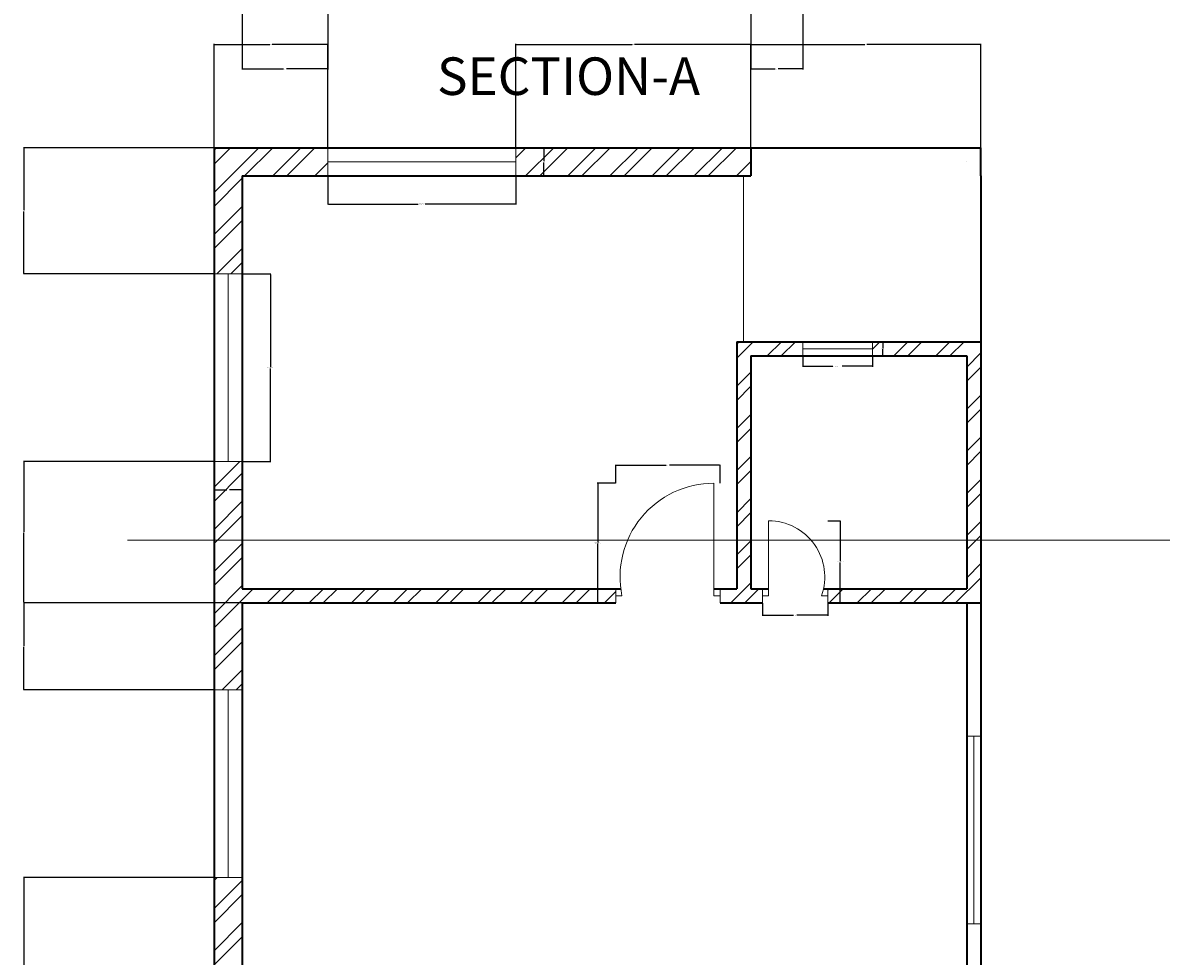
# Model space of a CAD drawing. Units: inches. Extents: x 1850 to 3445, y 1558 to 2756.
# Tile 10 of 13: x 2640 to 3003, y 1958 to 2256. Entities that reach past the tile are written whole.
import ezdxf

# ---------------------------------------------------------------- set-up
doc = ezdxf.new("R2010")
doc.units = ezdxf.units.IN
for name, color, linetype, lineweight in [('A-ANNO-DIMS', 2, 'Continuous', 18), ('A-ANNO-SYMB', 2, 'Continuous', 18), ('A-ANNO-TEXT', 7, 'Continuous', 18), ('A-DOOR', 3, 'Continuous', 18), ('A-GLAZ', 4, 'Continuous', 18), ('A-WALL', 7, 'Continuous', 35), ('A-WALL-PATT', 252, 'Continuous', 13)]:
    doc.layers.add(name, color=color, linetype=linetype, lineweight=lineweight)
doc.styles.get("Standard").update_dxf_attribs({"font": 'arial.ttf'})
doc.dimstyles.get("Standard").update_dxf_attribs({"dimtxt": 0.18, "dimasz": 0.18, "dimexe": 0.18, "dimexo": 0.0625, "dimgap": 0.09, "dimtad": 0, "dimtih": 1, "dimtoh": 1, "dimdec": 4, "dimzin": 0, "dimdsep": 46, "dimtxsty": 'Standard', "dimcen": 0.09, "dimadec": 0, "dimazin": 0, "dimtfac": 1, "dimtdec": 4, "dimtofl": 0, "dimtmove": 0, "dimatfit": 3, "dimfxl": 1, "dimtolj": 1, "dimtzin": 0, "dimarcsym": 0})

# ---------------------------------------------------------------- blocks, each defined once
blk = doc.blocks.new('WIN-60-W9')
for p, q in [((0, 9), (0, 0)), ((60, 4.5), (60, 9)), ((60, 9), (60, 0)), ((0, 0), (0, 4.5)), ((0, 4.5), (60, 4.5))]:
    blk.add_line(p, q)
blk = doc.blocks.new('WIN-60-W9-ALT')
for p, q in [((9, 60), (0, 60)), ((0, 60), (4.5, 60)), ((4.5, 60), (4.5, 0)), ((4.5, 0), (0, 0)), ((0, 0), (9, 0))]:
    blk.add_line(p, q)
blk = doc.blocks.new('WIN-60-W4_5')
for p, q in [((0, 60), (4.5, 60)), ((4.5, 60), (2.25, 60)), ((2.25, 60), (2.25, 0)), ((2.25, 0), (0, 0)), ((0, 0), (4.5, 0))]:
    blk.add_line(p, q)
blk = doc.blocks.new('WIN-BATH-GROUND')
for p, q in [((0, 0), (0, 4.5)), ((22.27, 2.25), (22.27, 4.5)), ((22.27, 4.5), (22.27, 0)), ((0, 2.25), (22.27, 2.25))]:
    blk.add_line(p, q)
blk = doc.blocks.new('DOOR-BATH-GROUND')
for p, q in [((2, 2.25), (2, 26.25)), ((0, 4.5), (0, 0)), ((20.9, 4.5), (20.9, 0)), ((0, 0), (0, 2.25)), ((0, 2.25), (2, 2.25)), ((20.9, 2.25), (18.9, 2.25)), ((20.9, 0), (20.9, 2.25))]:
    blk.add_line(p, q)
blk.add_arc((2, 8.3), 17.95, 340.2941, 90)
blk = doc.blocks.new('DOOR-BED-GROUND')
for p, q in [((31.38, 2.25), (31.38, 38.25)), ((0, 4.5), (0, 0)), ((33.38, 4.5), (33.38, 0)), ((0, 0), (0, 2.25)), ((0, 2.25), (2, 2.25)), ((33.38, 2.25), (31.38, 2.25)), ((33.38, 0), (33.38, 2.25))]:
    blk.add_line(p, q)
blk.add_arc((31.38, 8.26), 29.99, 90, 191.5706)
blk = doc.blocks.new('*D28')
at = {"layer": 'A-ANNO-DIMS', "color": 0, "lineweight": -2, "transparency": 16777216}
for p, q in [((2737.2, 2207.12), (2737.2, 2198)), ((2797.2, 2207.12), (2797.2, 2198)), ((2737.38, 2198.18), (2766.08, 2198.18)), ((2797.02, 2198.18), (2768.32, 2198.18))]:
    blk.add_line(p, q, dxfattribs=at)
at = {"layer": 'A-ANNO-DIMS', "color": 0, "transparency": 16777216}
for points in [[(2737.38, 2198.21), (2737.38, 2198.15), (2737.2, 2198.18)], [(2797.02, 2198.21), (2797.02, 2198.15), (2797.2, 2198.18)]]:
    blk.add_solid(points, dxfattribs=at)
at = {"layer": 'Defpoints', "color": 0, "transparency": 16777216}
for p in [(2737.2, 2207.18), (2797.2, 2207.18), (2797.2, 2198.18)]:
    blk.add_point(p, dxfattribs=at)
at = {"layer": 'A-ANNO-DIMS', "color": 0, "transparency": 16777216, "insert": (2767.2, 2198.18), "char_height": 0.18, "attachment_point": 5}
blk.add_mtext('\\A1;WINDOW 60 TYP.', dxfattribs=at)
blk = doc.blocks.new('*D29')
at = {"layer": 'A-ANNO-DIMS', "color": 0, "lineweight": -2, "transparency": 16777216}
for p, q in [((2797.26, 2216.18), (2806.38, 2216.18)), ((2806.2, 2216), (2806.2, 2211.87)), ((2806.2, 2207.36), (2806.2, 2211.5)), ((2797.26, 2207.18), (2806.38, 2207.18))]:
    blk.add_line(p, q, dxfattribs=at)
at = {"layer": 'A-ANNO-DIMS', "color": 0, "transparency": 16777216}
for points in [[(2806.17, 2216), (2806.23, 2216), (2806.2, 2216.18)], [(2806.17, 2207.36), (2806.23, 2207.36), (2806.2, 2207.18)]]:
    blk.add_solid(points, dxfattribs=at)
at = {"layer": 'Defpoints', "color": 0, "transparency": 16777216}
for p in [(2797.2, 2216.18), (2806.2, 2216.18), (2797.2, 2207.18)]:
    blk.add_point(p, dxfattribs=at)
at = {"layer": 'A-ANNO-DIMS', "color": 0, "transparency": 16777216, "insert": (2806.2, 2211.68), "char_height": 0.18, "attachment_point": 5}
blk.add_mtext('\\A1;9 TYP.', dxfattribs=at)
blk = doc.blocks.new('*D32')
at = {"layer": 'A-ANNO-DIMS', "color": 0, "lineweight": -2, "transparency": 16777216}
for p, q in [((2709.88, 2175.83), (2719, 2175.83)), ((2718.82, 2175.65), (2718.82, 2146.01)), ((2718.82, 2116.01), (2718.82, 2145.65)), ((2709.88, 2115.83), (2719, 2115.83))]:
    blk.add_line(p, q, dxfattribs=at)
at = {"layer": 'A-ANNO-DIMS', "color": 0, "transparency": 16777216}
for points in [[(2718.79, 2175.65), (2718.85, 2175.65), (2718.82, 2175.83)], [(2718.79, 2116.01), (2718.85, 2116.01), (2718.82, 2115.83)]]:
    blk.add_solid(points, dxfattribs=at)
at = {"layer": 'Defpoints', "color": 0, "transparency": 16777216}
for p in [(2709.82, 2175.83), (2718.82, 2175.83), (2709.82, 2115.83)]:
    blk.add_point(p, dxfattribs=at)
at = {"layer": 'A-ANNO-DIMS', "color": 0, "transparency": 16777216, "insert": (2718.82, 2145.83), "char_height": 0.18, "attachment_point": 5}
blk.add_mtext('\\A1;WINDOW 60 TYP.', dxfattribs=at)
blk = doc.blocks.new('*D33')
at = {"layer": 'A-ANNO-DIMS', "color": 0, "lineweight": -2, "transparency": 16777216}
for p, q in [((2700.82, 2115.77), (2700.82, 2106.65)), ((2709.82, 2115.77), (2709.82, 2106.65)), ((2701, 2106.83), (2704.86, 2106.83)), ((2709.64, 2106.83), (2705.78, 2106.83))]:
    blk.add_line(p, q, dxfattribs=at)
at = {"layer": 'A-ANNO-DIMS', "color": 0, "transparency": 16777216}
for points in [[(2701, 2106.86), (2701, 2106.8), (2700.82, 2106.83)], [(2709.64, 2106.86), (2709.64, 2106.8), (2709.82, 2106.83)]]:
    blk.add_solid(points, dxfattribs=at)
at = {"layer": 'Defpoints', "color": 0, "transparency": 16777216}
for p in [(2700.82, 2115.83), (2709.82, 2115.83), (2709.82, 2106.83)]:
    blk.add_point(p, dxfattribs=at)
at = {"layer": 'A-ANNO-DIMS', "color": 0, "transparency": 16777216, "insert": (2705.32, 2106.83), "char_height": 0.18, "attachment_point": 5}
blk.add_mtext('\\A1;9 TYP.', dxfattribs=at)
blk = doc.blocks.new('*D44')
at = {"layer": 'A-ANNO-DIMS', "color": 0, "lineweight": -2, "transparency": 16777216}
for p, q in [((2888.9, 2149.62), (2888.9, 2146.16)), ((2889.08, 2146.34), (2898.55, 2146.34)), ((2910.99, 2146.34), (2901.51, 2146.34)), ((2911.17, 2149.62), (2911.17, 2146.16))]:
    blk.add_line(p, q, dxfattribs=at)
at = {"layer": 'A-ANNO-DIMS', "color": 0, "transparency": 16777216}
for points in [[(2889.08, 2146.37), (2889.08, 2146.31), (2888.9, 2146.34)], [(2910.99, 2146.37), (2910.99, 2146.31), (2911.17, 2146.34)]]:
    blk.add_solid(points, dxfattribs=at)
at = {"layer": 'Defpoints', "color": 0, "transparency": 16777216}
for p in [(2888.9, 2149.68), (2911.17, 2149.68), (2911.17, 2146.34)]:
    blk.add_point(p, dxfattribs=at)
at = {"layer": 'A-ANNO-DIMS', "color": 0, "transparency": 16777216, "insert": (2900.03, 2146.34), "char_height": 0.18, "attachment_point": 5}
blk.add_mtext('\\A1;BATH WINDOW 22 TYP.', dxfattribs=at)
blk = doc.blocks.new('*D45')
at = {"layer": 'A-ANNO-DIMS', "color": 0, "lineweight": -2, "transparency": 16777216}
for p, q in [((2911.23, 2154.18), (2914.69, 2154.18)), ((2914.51, 2154), (2914.51, 2152.12)), ((2914.51, 2149.86), (2914.51, 2151.75)), ((2911.23, 2149.68), (2914.69, 2149.68))]:
    blk.add_line(p, q, dxfattribs=at)
at = {"layer": 'A-ANNO-DIMS', "color": 0, "transparency": 16777216}
for points in [[(2914.48, 2154), (2914.54, 2154), (2914.51, 2154.18)], [(2914.48, 2149.86), (2914.54, 2149.86), (2914.51, 2149.68)]]:
    blk.add_solid(points, dxfattribs=at)
at = {"layer": 'Defpoints', "color": 0, "transparency": 16777216}
for p in [(2911.17, 2154.18), (2914.51, 2154.18), (2911.17, 2149.68)]:
    blk.add_point(p, dxfattribs=at)
at = {"layer": 'A-ANNO-DIMS', "color": 0, "transparency": 16777216, "insert": (2914.51, 2151.93), "char_height": 0.18, "attachment_point": 5}
blk.add_mtext('\\A1;5 TYP.', dxfattribs=at)
blk = doc.blocks.new('*D56')
at = {"layer": 'A-ANNO-DIMS', "color": 0, "lineweight": -2, "transparency": 16777216}
for p, q in [((2896.98, 2096.93), (2901.03, 2096.93)), ((2900.85, 2096.75), (2900.85, 2083.99)), ((2900.85, 2070.86), (2900.85, 2083.63)), ((2896.98, 2070.68), (2901.03, 2070.68))]:
    blk.add_line(p, q, dxfattribs=at)
at = {"layer": 'A-ANNO-DIMS', "color": 0, "transparency": 16777216}
for points in [[(2900.82, 2096.75), (2900.88, 2096.75), (2900.85, 2096.93)], [(2900.82, 2070.86), (2900.88, 2070.86), (2900.85, 2070.68)]]:
    blk.add_solid(points, dxfattribs=at)
at = {"layer": 'Defpoints', "color": 0, "transparency": 16777216}
for p in [(2896.91, 2096.93), (2900.85, 2096.93), (2896.91, 2070.68)]:
    blk.add_point(p, dxfattribs=at)
at = {"layer": 'A-ANNO-DIMS', "color": 0, "transparency": 16777216, "insert": (2900.85, 2083.81), "char_height": 0.18, "attachment_point": 5}
blk.add_mtext('\\A1;BATH DOOR 26 TYP.', dxfattribs=at)
blk = doc.blocks.new('*D57')
at = {"layer": 'A-ANNO-DIMS', "color": 0, "lineweight": -2, "transparency": 16777216}
for p, q in [((2876.02, 2070.62), (2876.02, 2066.57)), ((2896.91, 2070.62), (2896.91, 2066.57)), ((2876.2, 2066.75), (2885.94, 2066.75)), ((2896.73, 2066.75), (2886.99, 2066.75))]:
    blk.add_line(p, q, dxfattribs=at)
at = {"layer": 'A-ANNO-DIMS', "color": 0, "transparency": 16777216}
for points in [[(2876.2, 2066.78), (2876.2, 2066.72), (2876.02, 2066.75)], [(2896.73, 2066.78), (2896.73, 2066.72), (2896.91, 2066.75)]]:
    blk.add_solid(points, dxfattribs=at)
at = {"layer": 'Defpoints', "color": 0, "transparency": 16777216}
for p in [(2876.02, 2070.68), (2896.91, 2070.68), (2896.91, 2066.75)]:
    blk.add_point(p, dxfattribs=at)
at = {"layer": 'A-ANNO-DIMS', "color": 0, "transparency": 16777216, "insert": (2886.47, 2066.75), "char_height": 0.18, "attachment_point": 5}
blk.add_mtext('\\A1;21 TYP.', dxfattribs=at)
blk = doc.blocks.new('*D58')
at = {"layer": 'A-ANNO-DIMS', "color": 0, "lineweight": -2, "transparency": 16777216}
for p, q in [((2829.09, 2108.93), (2823.24, 2108.93)), ((2823.42, 2108.75), (2823.42, 2089.99)), ((2823.42, 2070.86), (2823.42, 2089.63)), ((2829.09, 2070.68), (2823.24, 2070.68))]:
    blk.add_line(p, q, dxfattribs=at)
at = {"layer": 'A-ANNO-DIMS', "color": 0, "transparency": 16777216}
for points in [[(2823.39, 2108.75), (2823.45, 2108.75), (2823.42, 2108.93)], [(2823.39, 2070.86), (2823.45, 2070.86), (2823.42, 2070.68)]]:
    blk.add_solid(points, dxfattribs=at)
at = {"layer": 'Defpoints', "color": 0, "transparency": 16777216}
for p in [(2823.42, 2108.93), (2829.16, 2108.93), (2829.16, 2070.68)]:
    blk.add_point(p, dxfattribs=at)
at = {"layer": 'A-ANNO-DIMS', "color": 0, "transparency": 16777216, "insert": (2823.42, 2089.81), "char_height": 0.18, "attachment_point": 5}
blk.add_mtext('\\A1;BED DOOR 38 TYP.', dxfattribs=at)
blk = doc.blocks.new('*D59')
at = {"layer": 'A-ANNO-DIMS', "color": 0, "lineweight": -2, "transparency": 16777216}
for p, q in [((2829.16, 2109), (2829.16, 2114.85)), ((2829.34, 2114.67), (2845.32, 2114.67)), ((2862.35, 2114.67), (2846.37, 2114.67)), ((2862.53, 2109), (2862.53, 2114.85))]:
    blk.add_line(p, q, dxfattribs=at)
at = {"layer": 'A-ANNO-DIMS', "color": 0, "transparency": 16777216}
for points in [[(2829.34, 2114.7), (2829.34, 2114.64), (2829.16, 2114.67)], [(2862.35, 2114.7), (2862.35, 2114.64), (2862.53, 2114.67)]]:
    blk.add_solid(points, dxfattribs=at)
at = {"layer": 'Defpoints', "color": 0, "transparency": 16777216}
for p in [(2862.53, 2114.67), (2829.16, 2108.93), (2862.53, 2108.93)]:
    blk.add_point(p, dxfattribs=at)
at = {"layer": 'A-ANNO-DIMS', "color": 0, "transparency": 16777216, "insert": (2845.84, 2114.67), "char_height": 0.18, "attachment_point": 5}
blk.add_mtext('\\A1;33 TYP.', dxfattribs=at)
blk = doc.blocks.new('*D86')
at = {"layer": 'A-ANNO-DIMS', "color": 0, "lineweight": -2, "transparency": 16777216}
for p, q in [((2700.82, 2216.25), (2700.82, 2249.41)), ((2701, 2249.23), (2718.62, 2249.23)), ((2737.02, 2249.23), (2719.4, 2249.23)), ((2737.2, 2216.25), (2737.2, 2249.41))]:
    blk.add_line(p, q, dxfattribs=at)
at = {"layer": 'A-ANNO-DIMS', "color": 0, "transparency": 16777216}
for points in [[(2701, 2249.26), (2701, 2249.2), (2700.82, 2249.23)], [(2737.02, 2249.26), (2737.02, 2249.2), (2737.2, 2249.23)]]:
    blk.add_solid(points, dxfattribs=at)
at = {"layer": 'Defpoints', "color": 0, "transparency": 16777216}
for p in [(2737.2, 2249.23), (2700.82, 2216.18), (2737.2, 2216.18)]:
    blk.add_point(p, dxfattribs=at)
at = {"layer": 'A-ANNO-DIMS', "color": 0, "transparency": 16777216, "insert": (2719.01, 2249.23), "char_height": 0.18, "attachment_point": 5}
blk.add_mtext('\\A1;36.38', dxfattribs=at)
blk = doc.blocks.new('*D87')
at = {"layer": 'A-ANNO-DIMS', "color": 0, "lineweight": -2, "transparency": 16777216}
for p, q in [((2797.2, 2216.25), (2797.2, 2249.41)), ((2797.38, 2249.23), (2834.37, 2249.23)), ((2872.14, 2249.23), (2835.15, 2249.23)), ((2872.32, 2216.25), (2872.32, 2249.41))]:
    blk.add_line(p, q, dxfattribs=at)
at = {"layer": 'A-ANNO-DIMS', "color": 0, "transparency": 16777216}
for points in [[(2797.38, 2249.26), (2797.38, 2249.2), (2797.2, 2249.23)], [(2872.14, 2249.26), (2872.14, 2249.2), (2872.32, 2249.23)]]:
    blk.add_solid(points, dxfattribs=at)
at = {"layer": 'Defpoints', "color": 0, "transparency": 16777216}
for p in [(2872.32, 2249.23), (2797.2, 2216.18), (2872.32, 2216.18)]:
    blk.add_point(p, dxfattribs=at)
at = {"layer": 'A-ANNO-DIMS', "color": 0, "transparency": 16777216, "insert": (2834.76, 2249.23), "char_height": 0.18, "attachment_point": 5}
blk.add_mtext('\\A1;75.12', dxfattribs=at)
blk = doc.blocks.new('*D88')
at = {"layer": 'A-ANNO-DIMS', "color": 0, "lineweight": -2, "transparency": 16777216}
for p, q in [((2872.32, 2216.25), (2872.32, 2249.41)), ((2872.5, 2249.23), (2908.75, 2249.23)), ((2945.64, 2249.23), (2909.4, 2249.23)), ((2945.82, 2216.25), (2945.82, 2249.41))]:
    blk.add_line(p, q, dxfattribs=at)
at = {"layer": 'A-ANNO-DIMS', "color": 0, "transparency": 16777216}
for points in [[(2872.5, 2249.26), (2872.5, 2249.2), (2872.32, 2249.23)], [(2945.64, 2249.26), (2945.64, 2249.2), (2945.82, 2249.23)]]:
    blk.add_solid(points, dxfattribs=at)
at = {"layer": 'Defpoints', "color": 0, "transparency": 16777216}
for p in [(2945.82, 2249.23), (2872.32, 2216.18), (2945.82, 2216.18)]:
    blk.add_point(p, dxfattribs=at)
at = {"layer": 'A-ANNO-DIMS', "color": 0, "transparency": 16777216, "insert": (2909.07, 2249.23), "char_height": 0.18, "attachment_point": 5}
blk.add_mtext('\\A1;73.5', dxfattribs=at)
blk = doc.blocks.new('*D98')
at = {"layer": 'A-ANNO-DIMS', "color": 0, "lineweight": -2, "transparency": 16777216}
for p, q in [((2700.76, 1982.85), (2639.89, 1982.85)), ((2640.07, 1982.67), (2640.07, 1946.71)), ((2640.07, 1910.4), (2640.07, 1946.35)), ((2700.76, 1910.22), (2639.89, 1910.22))]:
    blk.add_line(p, q, dxfattribs=at)
at = {"layer": 'A-ANNO-DIMS', "color": 0, "transparency": 16777216}
for points in [[(2640.04, 1982.67), (2640.1, 1982.67), (2640.07, 1982.85)], [(2640.04, 1910.4), (2640.1, 1910.4), (2640.07, 1910.22)]]:
    blk.add_solid(points, dxfattribs=at)
at = {"layer": 'Defpoints', "color": 0, "transparency": 16777216}
for p in [(2640.07, 1982.85), (2700.82, 1982.85), (2700.82, 1910.22)]:
    blk.add_point(p, dxfattribs=at)
at = {"layer": 'A-ANNO-DIMS', "color": 0, "transparency": 16777216, "insert": (2640.07, 1946.53), "char_height": 0.18, "attachment_point": 5}
blk.add_mtext('\\A1;72.63', dxfattribs=at)
blk = doc.blocks.new('*D99')
at = {"layer": 'A-ANNO-DIMS', "color": 0, "lineweight": -2, "transparency": 16777216}
for p, q in [((2709.76, 2070.68), (2639.89, 2070.68)), ((2640.07, 2070.5), (2640.07, 2056.95)), ((2640.07, 2043.03), (2640.07, 2056.58)), ((2700.76, 2042.85), (2639.89, 2042.85))]:
    blk.add_line(p, q, dxfattribs=at)
at = {"layer": 'A-ANNO-DIMS', "color": 0, "transparency": 16777216}
for points in [[(2640.04, 2070.5), (2640.1, 2070.5), (2640.07, 2070.68)], [(2640.04, 2043.03), (2640.1, 2043.03), (2640.07, 2042.85)]]:
    blk.add_solid(points, dxfattribs=at)
at = {"layer": 'Defpoints', "color": 0, "transparency": 16777216}
for p in [(2640.07, 2070.68), (2709.82, 2070.68), (2700.82, 2042.85)]:
    blk.add_point(p, dxfattribs=at)
at = {"layer": 'A-ANNO-DIMS', "color": 0, "transparency": 16777216, "insert": (2640.07, 2056.77), "char_height": 0.18, "attachment_point": 5}
blk.add_mtext('\\A1;27.84', dxfattribs=at)
blk = doc.blocks.new('*D100')
at = {"layer": 'A-ANNO-DIMS', "color": 0, "lineweight": -2, "transparency": 16777216}
for p, q in [((2700.76, 2115.83), (2639.89, 2115.83)), ((2640.07, 2115.65), (2640.07, 2093.44)), ((2640.07, 2070.86), (2640.07, 2093.08)), ((2709.76, 2070.68), (2639.89, 2070.68))]:
    blk.add_line(p, q, dxfattribs=at)
at = {"layer": 'A-ANNO-DIMS', "color": 0, "transparency": 16777216}
for points in [[(2640.04, 2115.65), (2640.1, 2115.65), (2640.07, 2115.83)], [(2640.04, 2070.86), (2640.1, 2070.86), (2640.07, 2070.68)]]:
    blk.add_solid(points, dxfattribs=at)
at = {"layer": 'Defpoints', "color": 0, "transparency": 16777216}
for p in [(2640.07, 2115.83), (2700.82, 2115.83), (2709.82, 2070.68)]:
    blk.add_point(p, dxfattribs=at)
at = {"layer": 'A-ANNO-DIMS', "color": 0, "transparency": 16777216, "insert": (2640.07, 2093.26), "char_height": 0.18, "attachment_point": 5}
blk.add_mtext('\\A1;45.15', dxfattribs=at)
blk = doc.blocks.new('*D101')
at = {"layer": 'A-ANNO-DIMS', "color": 0, "lineweight": -2, "transparency": 16777216}
for p, q in [((2700.76, 2216.18), (2639.89, 2216.18)), ((2640.07, 2216), (2640.07, 2196.19)), ((2640.07, 2176.01), (2640.07, 2195.83)), ((2700.76, 2175.83), (2639.89, 2175.83))]:
    blk.add_line(p, q, dxfattribs=at)
at = {"layer": 'A-ANNO-DIMS', "color": 0, "transparency": 16777216}
for points in [[(2640.04, 2216), (2640.1, 2216), (2640.07, 2216.18)], [(2640.04, 2176.01), (2640.1, 2176.01), (2640.07, 2175.83)]]:
    blk.add_solid(points, dxfattribs=at)
at = {"layer": 'Defpoints', "color": 0, "transparency": 16777216}
for p in [(2640.07, 2216.18), (2700.82, 2216.18), (2700.82, 2175.83)]:
    blk.add_point(p, dxfattribs=at)
at = {"layer": 'A-ANNO-DIMS', "color": 0, "transparency": 16777216, "insert": (2640.07, 2196.01), "char_height": 0.18, "attachment_point": 5}
blk.add_mtext('\\A1;40.354', dxfattribs=at)
blk = doc.blocks.new('*D124')
at = {"layer": 'A-ANNO-DIMS', "color": 0, "lineweight": -2, "transparency": 16777216}
for p, q in [((2737.2, 2316.81), (2737.2, 2241.19)), ((2709.82, 2280.81), (2709.82, 2241.19)), ((2710, 2241.37), (2723.05, 2241.37)), ((2737.02, 2241.37), (2723.98, 2241.37))]:
    blk.add_line(p, q, dxfattribs=at)
at = {"layer": 'A-ANNO-DIMS', "color": 0, "transparency": 16777216}
for points in [[(2710, 2241.4), (2710, 2241.34), (2709.82, 2241.37)], [(2737.02, 2241.4), (2737.02, 2241.34), (2737.2, 2241.37)]]:
    blk.add_solid(points, dxfattribs=at)
at = {"layer": 'Defpoints', "color": 0, "transparency": 16777216}
for p in [(2737.2, 2316.87), (2709.82, 2280.87), (2737.2, 2241.37)]:
    blk.add_point(p, dxfattribs=at)
at = {"layer": 'A-ANNO-DIMS', "color": 0, "transparency": 16777216, "insert": (2723.51, 2241.37), "char_height": 0.18, "attachment_point": 5}
blk.add_mtext('\\A1;27.377', dxfattribs=at)
blk = doc.blocks.new('*D125')
at = {"layer": 'A-ANNO-DIMS', "color": 0, "lineweight": -2, "transparency": 16777216}
for p, q in [((2888.9, 2316.81), (2888.9, 2241.19)), ((2872.32, 2280.81), (2872.32, 2241.19)), ((2872.5, 2241.37), (2880.16, 2241.37)), ((2888.72, 2241.37), (2881.07, 2241.37))]:
    blk.add_line(p, q, dxfattribs=at)
at = {"layer": 'A-ANNO-DIMS', "color": 0, "transparency": 16777216}
for points in [[(2872.5, 2241.4), (2872.5, 2241.34), (2872.32, 2241.37)], [(2888.72, 2241.4), (2888.72, 2241.34), (2888.9, 2241.37)]]:
    blk.add_solid(points, dxfattribs=at)
at = {"layer": 'Defpoints', "color": 0, "transparency": 16777216}
for p in [(2888.9, 2316.87), (2872.32, 2280.87), (2888.9, 2241.37)]:
    blk.add_point(p, dxfattribs=at)
at = {"layer": 'A-ANNO-DIMS', "color": 0, "transparency": 16777216, "insert": (2880.61, 2241.37), "char_height": 0.18, "attachment_point": 5}
blk.add_mtext('\\A1;16.577', dxfattribs=at)

msp = doc.modelspace()

# ---------------------------------------------------------------- hatches: boundary and pattern name
at = {"layer": 'A-WALL-PATT'}
h = msp.add_hatch(dxfattribs=at)
h.set_pattern_fill('ANSI32', color=256)
h.set_pattern_definition([(45, (660.551, 0), (-6.735192, 6.735192), []), (45, (665.041, 0), (-6.735192, 6.735192), [])])
h.paths.add_polyline_path([(3180.1061, 1907.3936), (3184.5492, 1907.3936), (3184.5492, 1916.3936), (3180.1061, 1916.3936), (3175.6061, 1916.3936), (3171.1061, 1916.3936), (3171.1061, 1907.3936), (3175.6061, 1907.3936), (3175.6061, 1742.1843), (3175.6061, 1737.6843), (3256.6061, 1737.6843), (3256.6061, 1976.4962), (3252.1061, 1976.4962), (3252.1061, 1916.3936), (3221.8172, 1916.3936), (3221.8172, 1907.3936), (3252.1061, 1907.3936), (3252.1061, 1746.6843), (3180.1061, 1746.6843)])
h.paths.add_polyline_path([(2737.1986, 2211.6843), (2737.1986, 2216.1843), (2700.822, 2216.1843), (2700.822, 2175.83), (2705.322, 2175.83), (2709.822, 2175.83), (2709.822, 2207.1843), (2737.1986, 2207.1843)])
h.paths.add_polyline_path([(2872.322, 2216.1843), (2797.1986, 2216.1843), (2797.1986, 2207.1843), (2872.322, 2207.1843)])
h.paths.add_polyline_path([(2945.822, 2154.1843), (2911.1674, 2154.1843), (2911.1674, 2149.6843), (2941.322, 2149.6843), (2941.322, 2075.1843), (2896.9138, 2075.1843), (2896.9138, 2070.6843), (2945.822, 2070.6843)])
h.paths.add_polyline_path([(2888.8991, 2154.1843), (2867.822, 2154.1843), (2867.822, 2075.1843), (2862.5325, 2075.1843), (2862.5325, 2070.6843), (2876.0169, 2070.6843), (2876.0169, 2072.9343), (2876.0169, 2075.1843), (2872.322, 2075.1843), (2872.322, 2149.6843), (2888.8991, 2149.6843)])
h.paths.add_polyline_path([(2709.822, 2115.83), (2700.822, 2115.83), (2700.822, 2042.8465), (2709.822, 2042.8465), (2709.822, 2070.6843), (2829.1562, 2070.6843), (2829.1562, 2072.9343), (2829.1562, 2075.1843), (2709.822, 2075.1843)])
h.paths.add_polyline_path([(2709.822, 1982.8465), (2700.822, 1982.8465), (2700.822, 1910.2175), (2721.4986, 1910.2175), (2721.4986, 1914.7175), (2721.4986, 1919.2175), (2709.822, 1919.2175)])
h.paths.add_polyline_path([(2793.0443, 1919.2175), (2769.4986, 1919.2175), (2769.4986, 1910.2175), (2793.0443, 1910.2175), (2793.0443, 1914.6749)])
h.paths.add_polyline_path([(2839.322, 1938.6843), (2830.322, 1938.6843), (2830.322, 1919.2175), (2824.2376, 1919.2175), (2824.2376, 1910.2175), (2830.322, 1910.2175), (2830.322, 1854.6843), (2830.322, 1845.6843), (2856.6792, 1845.6843), (2856.6792, 1850.1843), (2856.6792, 1854.6843), (2839.322, 1854.6843)])
h.paths.add_polyline_path([(2709.822, 1910.2175), (2700.822, 1910.2175), (2700.822, 1745.6843), (2709.822, 1745.6843)])
h.paths.add_polyline_path([(2807.4367, 1766.7204), (2819.64, 1766.7204), (2819.64, 1777.0239), (2807.4367, 1777.0239)], flags=9)
h.paths.add_polyline_path([(2844.0169, 1798.4016), (2887.2843, 1798.4016), (2887.2843, 1817.0589), (2844.0169, 1817.0589)], flags=9)
h.paths.add_polyline_path([(2731.4135, 1867.537), (2770.5302, 1867.537), (2770.5302, 1886.1943), (2731.4135, 1886.1943)], flags=9)

# ---------------------------------------------------------------- linework, layer by layer
at = {"layer": 'A-ANNO-SYMB'}
msp.add_line((2673.1156, 2090.7612), (3313.7387, 2090.7612), dxfattribs=at)
at = {"layer": 'A-GLAZ'}
msp.add_line((2870.0024, 2207.1843), (2870.0024, 2154.1843), dxfattribs=at)
at = {"layer": 'A-WALL'}
for p, q in [((2700.822, 2216.1843), (2945.822, 2216.1843)), ((2700.822, 2216.1843), (2700.822, 1745.6843)), ((2872.322, 2216.1843), (2872.322, 2207.1843)), ((2945.822, 2207.1843), (2945.822, 2216.1843)), ((2941.295, 2211.8893), (2941.295, 2211.8893)), ((2709.822, 2207.1843), (2872.322, 2207.1843)), ((2709.822, 2207.1843), (2709.822, 2075.1843)), ((2945.822, 2207.1843), (2945.822, 1745.6843)), ((2867.822, 2154.1843), (2945.822, 2154.1843)), ((2867.822, 2154.1843), (2867.822, 2075.1843)), ((2872.322, 2149.6843), (2941.322, 2149.6843)), ((2872.322, 2149.6843), (2872.322, 2075.1843)), ((2941.322, 2149.6843), (2941.322, 2075.1843)), ((2709.822, 2075.1843), (2830.7841, 2075.1843)), ((2860.5325, 2075.1843), (2867.822, 2075.1843)), ((2872.322, 2075.1843), (2878.0169, 2075.1843)), ((2895.5576, 2075.1843), (2941.322, 2075.1843)), ((2709.822, 2070.6843), (2829.1562, 2070.6843)), ((2709.822, 2070.6843), (2709.822, 1919.2175)), ((2862.5325, 2070.6843), (2876.0169, 2070.6843)), ((2896.9138, 2070.6843), (2945.822, 2070.6843)), ((2941.322, 2070.6843), (2941.322, 1854.6843))]:
    msp.add_line(p, q, dxfattribs=at)

# ---------------------------------------------------------------- block references
at = {"layer": 'A-DOOR'}
for name, p in [('DOOR-BED-GROUND', (2829.1565, 2070.684)), ('DOOR-BATH-GROUND', (2876.0165, 2070.684))]:
    msp.add_blockref(name, p, dxfattribs=at)
at = {"layer": 'A-GLAZ'}
for name, p in [('WIN-60-W9', (2737.1985, 2207.184)), ('WIN-60-W9-ALT', (2700.8215, 2115.83)), ('WIN-BATH-GROUND', (2888.8995, 2149.684))]:
    msp.add_blockref(name, p, dxfattribs=at)
at = {"layer": 'A-GLAZ', "rotation": 90}
msp.add_blockref('WIN-60-W9', (2709.8223, 1982.8465), dxfattribs=at)
at = {"layer": 'A-GLAZ', "extrusion": (0, 0, -1), "zscale": -1}
msp.add_blockref('WIN-60-W4_5', (-2945.8225, 1968.032), dxfattribs=at)

# ---------------------------------------------------------------- texts
at = {"layer": 'A-ANNO-TEXT', "insert": (2772.0538, 2245.0592), "char_height": 12, "attachment_point": 1}
msp.add_mtext_dynamic_manual_height_columns('SECTION-A', width=159.205584, gutter_width=12.5, heights=[0], dxfattribs=at)

# ---------------------------------------------------------------- dimensions: what is measured, and where the dimension line sits
at = {"layer": 'A-ANNO-DIMS'}
for base, p1, p2, override, picture, middle in [((2737.1986, 2241.3737), (2709.822, 2280.8737), (2737.1986, 2316.8737), {"dimdec": 3, "dimlfac": 1, "dimrnd": 0, "dimzin": 0, "dimdsep": 46, "dimlunit": 2}, '*D124', (2723.5103, 2241.3737)), ((2888.8991, 2241.3737), (2872.322, 2280.8737), (2888.8991, 2316.8737), {"dimdec": 3, "dimlfac": 1, "dimrnd": 0, "dimzin": 0, "dimdsep": 46, "dimlunit": 2}, '*D125', (2880.6105, 2241.3737)), ((2737.1986, 2249.2343), (2700.822, 2216.1843), (2737.1986, 2216.1843), {"dimdec": 2, "dimlfac": 1, "dimrnd": 0, "dimzin": 0, "dimdsep": 46, "dimlunit": 2}, '*D86', (2719.0103, 2249.2343)), ((2872.322, 2249.2343), (2797.1986, 2216.1843), (2872.322, 2216.1843), {"dimdec": 2, "dimlfac": 1, "dimrnd": 0, "dimzin": 0, "dimdsep": 46, "dimlunit": 2}, '*D87', (2834.7603, 2249.2343)), ((2945.822, 2249.2343), (2872.322, 2216.1843), (2945.822, 2216.1843), {"dimdec": 1, "dimlfac": 1, "dimrnd": 0, "dimzin": 0, "dimdsep": 46, "dimlunit": 2}, '*D88', (2909.072, 2249.2343))]:
    dim = msp.add_linear_dim(base=base, p1=p1, p2=p2, dimstyle='Standard', override=override, dxfattribs=at)
    dim.commit()
    dim.dimension.update_dxf_attribs({"geometry": picture, "text_midpoint": middle})
for base, p1, p2, override, picture, middle in [((2640.0656, 2216.1843), (2700.822, 2175.83), (2700.822, 2216.1843), {"dimdec": 3, "dimlfac": 1, "dimrnd": 0, "dimzin": 0, "dimdsep": 46, "dimlunit": 2}, '*D101', (2640.0656, 2196.0071)), ((2640.0656, 2115.83), (2709.822, 2070.6843), (2700.822, 2115.83), {"dimdec": 2, "dimlfac": 1, "dimrnd": 0, "dimzin": 0, "dimdsep": 46, "dimlunit": 2}, '*D100', (2640.0656, 2093.2571)), ((2640.0656, 2070.6843), (2700.822, 2042.8465), (2709.822, 2070.6843), {"dimdec": 2, "dimlfac": 1, "dimrnd": 0, "dimzin": 0, "dimdsep": 46, "dimlunit": 2}, '*D99', (2640.0656, 2056.7654)), ((2640.0656, 1982.8465), (2700.822, 1910.2175), (2700.822, 1982.8465), {"dimdec": 2, "dimlfac": 1, "dimrnd": 0, "dimzin": 0, "dimdsep": 46, "dimlunit": 2}, '*D98', (2640.0656, 1946.532))]:
    dim = msp.add_linear_dim(base=base, p1=p1, p2=p2, angle=90, dimstyle='Standard', override=override, dxfattribs=at)
    dim.commit()
    dim.dimension.update_dxf_attribs({"geometry": picture, "text_midpoint": middle})
for base, p1, p2, text, picture, middle in [((2806.1986, 2216.1843), (2797.1986, 2207.1843), (2797.1986, 2216.1843), '<> TYP.', '*D29', (2806.1986, 2211.6843)), ((2718.822, 2175.83), (2709.822, 2115.83), (2709.822, 2175.83), 'WINDOW <> TYP.', '*D32', (2718.822, 2145.83)), ((2914.5076914886, 2154.1842850418), (2911.1674342354, 2149.6842850418), (2911.1674342354, 2154.1842850418), '<> TYP.', '*D45', (2914.5076914886, 2151.9342850418)), ((2823.4187, 2108.9343), (2829.1562, 2070.6843), (2829.1562, 2108.9343), 'BED DOOR <> TYP.', '*D58', (2823.4187, 2089.8093)), ((2900.8513, 2096.9343), (2896.9138, 2070.6843), (2896.9138, 2096.9343), 'BATH DOOR <> TYP.', '*D56', (2900.8513, 2083.8093))]:
    dim = msp.add_linear_dim(base=base, p1=p1, p2=p2, angle=90, text=text, dimstyle='Standard', override={"dimdec": 0, "dimlfac": 1, "dimrnd": 0, "dimzin": 0, "dimdsep": 46, "dimlunit": 2}, dxfattribs=at)
    dim.commit()
    dim.dimension.update_dxf_attribs({"geometry": picture, "text_midpoint": middle})
for base, p1, p2, text, picture, middle in [((2797.1986, 2198.1843), (2737.1986, 2207.1843), (2797.1986, 2207.1843), 'WINDOW <> TYP.', '*D28', (2767.1986, 2198.1843)), ((2911.1674, 2146.344), (2888.8991, 2149.6843), (2911.1674, 2149.6843), 'BATH WINDOW <> TYP.', '*D44', (2900.0332, 2146.344)), ((2709.822, 2106.83), (2700.822, 2115.83), (2709.822, 2115.83), '<> TYP.', '*D33', (2705.322, 2106.83)), ((2862.5325, 2114.6718), (2829.1562, 2108.9343), (2862.5325, 2108.9343), '<> TYP.', '*D59', (2845.8443, 2114.6718)), ((2896.9138, 2066.7468), (2876.0169, 2070.6843), (2896.9138, 2070.6843), '<> TYP.', '*D57', (2886.4653, 2066.7468))]:
    dim = msp.add_linear_dim(base=base, p1=p1, p2=p2, text=text, dimstyle='Standard', override={"dimdec": 0, "dimlfac": 1, "dimrnd": 0, "dimzin": 0, "dimdsep": 46, "dimlunit": 2}, dxfattribs=at)
    dim.commit()
    dim.dimension.update_dxf_attribs({"geometry": picture, "text_midpoint": middle})

doc.saveas('drawing.dxf')
